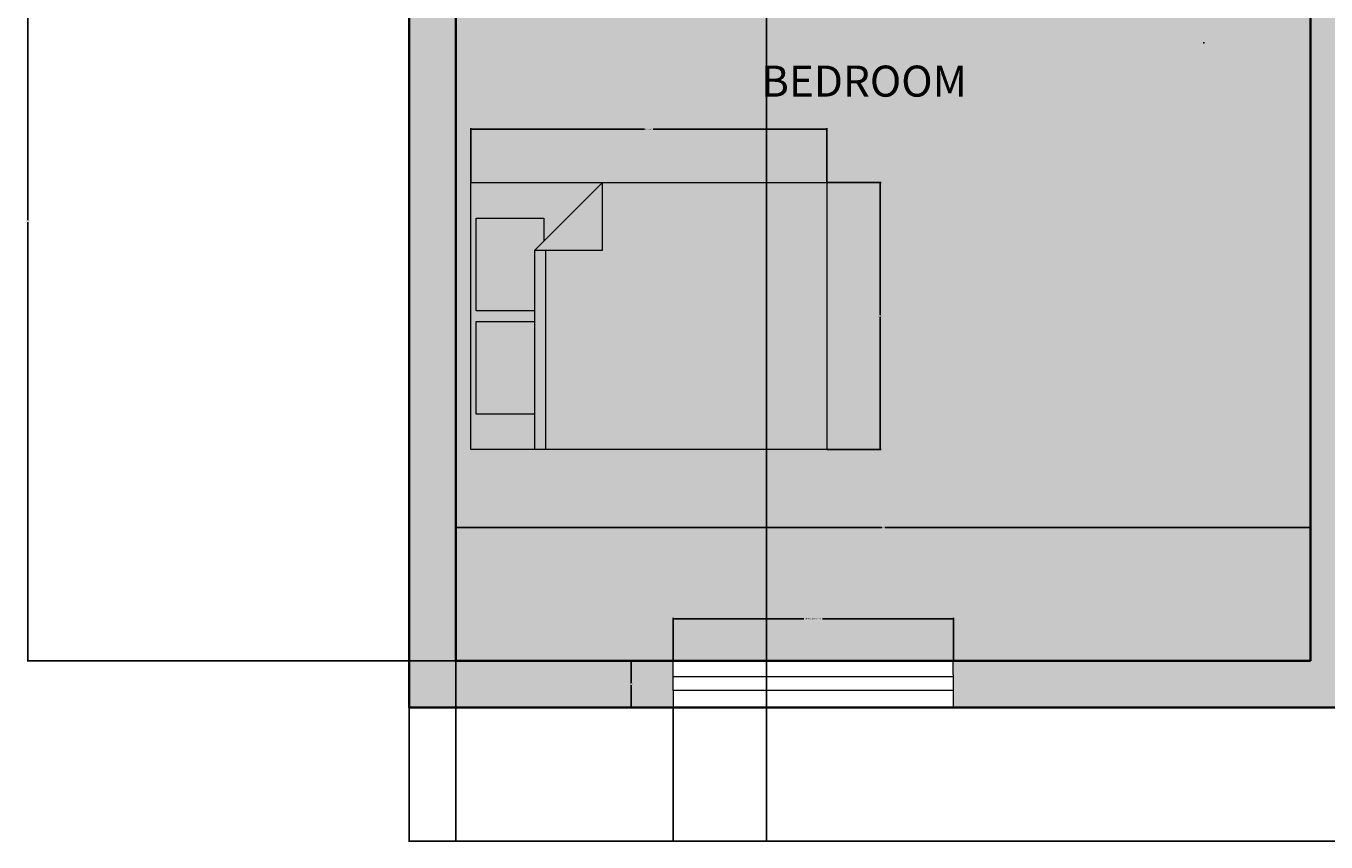
# Model space of a CAD drawing. Units: inches. Extents: x 3024 to 3952, y 1308 to 1863.
# Tile 1 of 29: x 3024 to 3275, y 1322 to 1479. Entities that reach past the tile are written whole.
import ezdxf

# ---------------------------------------------------------------- set-up
doc = ezdxf.new("R2010")
doc.units = ezdxf.units.IN
for name, color, linetype, lineweight in [('A-ANNO-DIMS', 2, 'Continuous', 18), ('A-AREA-IDEN', 7, 'Continuous', 18), ('A-FLOR-TILE-PATT', 7, 'Continuous', 13), ('A-FURN', 8, 'Continuous', 18), ('A-FURN-PATT', 9, 'Continuous', 13), ('A-GLAZ', 4, 'Continuous', 18), ('A-WALL', 7, 'Continuous', 35)]:
    doc.layers.add(name, color=color, linetype=linetype, lineweight=lineweight)
doc.layers.add('A-FLOR-PATT', color=254, linetype='Continuous', lineweight=13, true_color=0xfeeab9)
doc.layers.add('A-WALL-PATT', color=254, linetype='Continuous', lineweight=13, true_color=0xcecce6)
doc.styles.get("Standard").update_dxf_attribs({"font": 'arial.ttf'})
doc.dimstyles.get("Standard").update_dxf_attribs({"dimtxt": 0.18, "dimasz": 0.18, "dimexe": 0.18, "dimexo": 0.0625, "dimgap": 0.09, "dimtad": 0, "dimtih": 1, "dimtoh": 1, "dimdec": 4, "dimzin": 0, "dimdsep": 46, "dimtxsty": 'Standard', "dimcen": 0.09, "dimadec": 0, "dimazin": 0, "dimtfac": 1, "dimtdec": 4, "dimtofl": 0, "dimtmove": 0, "dimatfit": 3, "dimfxl": 1, "dimtolj": 1, "dimtzin": 0, "dimarcsym": 0})

# ---------------------------------------------------------------- blocks, each defined once
blk = doc.blocks.new('Bed - Queen')
for p, q in [((0, -80.00003), (0, 0)), ((0, 0), (59.99999, 0)), ((59.99999, 0), (59.99999, -80.00003)), ((7.99999, -1.2), (28.79998, -1.2)), ((7.99999, -14.4), (7.99999, -1.2)), ((28.79998, -1.2), (28.79998, -14.4)), ((31.19999, -1.2), (51.99999, -1.2)), ((31.19999, -14.4), (31.19999, -1.2)), ((51.99999, -1.2), (51.99999, -16.4)), ((0, -14.4), (44.8, -14.4)), ((59.99999, -29.6), (44.8, -14.4)), ((44.8, -14.4), (44.8, -29.6)), ((44.8, -16.8), (0, -16.8)), ((51.99999, -16.4), (46.79936, -16.4)), ((44.8, -29.6), (59.99999, -29.6)), ((59.99999, -80.00003), (0, -80.00003))]:
    blk.add_line(p, q)
blk = doc.blocks.new('WIN-BEDROOM-54IN')
for p, q in [((0, 5.99), (0, 9)), ((54.08, 6.41), (54.08, 9)), ((54.08, 6.41), (54.08, 5.99)), ((0, 3.28), (0, 0)), ((54.08, 3.69), (54.08, 0))]:
    blk.add_line(p, q)
blk.add_lwpolyline([(0, 5.99), (54.08, 5.99), (54.08, 3.28), (0, 3.28)], close=True)
blk = doc.blocks.new('*D16')
at = {"layer": 'A-ANNO-DIMS', "color": 0, "lineweight": -2, "transparency": 16777216}
for p, q in [((3109.65, 1449.25), (3109.65, 1459.68)), ((3109.83, 1459.5), (3143.2, 1459.5)), ((3178.2, 1459.5), (3144.83, 1459.5)), ((3178.38, 1449.25), (3178.38, 1459.68))]:
    blk.add_line(p, q, dxfattribs=at)
at = {"layer": 'A-ANNO-DIMS', "color": 0, "transparency": 16777216}
for points in [[(3109.83, 1459.53), (3109.83, 1459.47), (3109.65, 1459.5)], [(3178.2, 1459.53), (3178.2, 1459.47), (3178.38, 1459.5)]]:
    blk.add_solid(points, dxfattribs=at)
at = {"layer": 'Defpoints', "color": 0, "transparency": 16777216}
for p in [(3109.65, 1459.5), (3109.65, 1449.19), (3178.38, 1449.19)]:
    blk.add_point(p, dxfattribs=at)
at = {"layer": 'A-ANNO-DIMS', "color": 0, "transparency": 16777216, "insert": (3144.01, 1459.5), "char_height": 0.18, "attachment_point": 5}
blk.add_mtext('\\A1;BED 69 TYP.', dxfattribs=at)
blk = doc.blocks.new('*D17')
at = {"layer": 'A-ANNO-DIMS', "color": 0, "lineweight": -2, "transparency": 16777216}
for p, q in [((3178.44, 1449.19), (3188.87, 1449.19)), ((3188.69, 1449.01), (3188.69, 1423.6)), ((3188.69, 1397.82), (3188.69, 1423.23)), ((3178.44, 1397.64), (3188.87, 1397.64))]:
    blk.add_line(p, q, dxfattribs=at)
at = {"layer": 'A-ANNO-DIMS', "color": 0, "transparency": 16777216}
for points in [[(3188.66, 1449.01), (3188.72, 1449.01), (3188.69, 1449.19)], [(3188.66, 1397.82), (3188.72, 1397.82), (3188.69, 1397.64)]]:
    blk.add_solid(points, dxfattribs=at)
at = {"layer": 'Defpoints', "color": 0, "transparency": 16777216}
for p in [(3178.38, 1449.19), (3188.69, 1449.19), (3178.38, 1397.64)]:
    blk.add_point(p, dxfattribs=at)
at = {"layer": 'A-ANNO-DIMS', "color": 0, "transparency": 16777216, "insert": (3188.69, 1423.41), "char_height": 0.18, "attachment_point": 5}
blk.add_mtext('\\A1;52 TYP.', dxfattribs=at)
blk = doc.blocks.new('*D24')
at = {"layer": 'A-ANNO-DIMS', "color": 0, "lineweight": -2, "transparency": 16777216}
for p, q in [((3148.73, 1356.91), (3148.73, 1365.14)), ((3148.91, 1364.96), (3173.97, 1364.96)), ((3202.63, 1364.96), (3177.56, 1364.96)), ((3202.81, 1356.91), (3202.81, 1365.14))]:
    blk.add_line(p, q, dxfattribs=at)
at = {"layer": 'A-ANNO-DIMS', "color": 0, "transparency": 16777216}
for points in [[(3148.91, 1364.99), (3148.91, 1364.93), (3148.73, 1364.96)], [(3202.63, 1364.99), (3202.63, 1364.93), (3202.81, 1364.96)]]:
    blk.add_solid(points, dxfattribs=at)
at = {"layer": 'Defpoints', "color": 0, "transparency": 16777216}
for p in [(3202.81, 1364.96), (3148.73, 1356.85), (3202.81, 1356.85)]:
    blk.add_point(p, dxfattribs=at)
at = {"layer": 'A-ANNO-DIMS', "color": 0, "transparency": 16777216, "insert": (3175.77, 1364.96), "char_height": 0.18, "attachment_point": 5}
blk.add_mtext('\\A1;BEDROOM WINDOW 54 TYP.', dxfattribs=at)
blk = doc.blocks.new('*D25')
at = {"layer": 'A-ANNO-DIMS', "color": 0, "lineweight": -2, "transparency": 16777216}
for p, q in [((3148.66, 1356.85), (3140.43, 1356.85)), ((3140.61, 1356.67), (3140.61, 1352.53)), ((3140.61, 1348.03), (3140.61, 1352.16)), ((3148.66, 1347.85), (3140.43, 1347.85))]:
    blk.add_line(p, q, dxfattribs=at)
at = {"layer": 'A-ANNO-DIMS', "color": 0, "transparency": 16777216}
for points in [[(3140.58, 1356.67), (3140.64, 1356.67), (3140.61, 1356.85)], [(3140.58, 1348.03), (3140.64, 1348.03), (3140.61, 1347.85)]]:
    blk.add_solid(points, dxfattribs=at)
at = {"layer": 'Defpoints', "color": 0, "transparency": 16777216}
for p in [(3140.61, 1356.85), (3148.73, 1356.85), (3148.73, 1347.85)]:
    blk.add_point(p, dxfattribs=at)
at = {"layer": 'A-ANNO-DIMS', "color": 0, "transparency": 16777216, "insert": (3140.61, 1352.35), "char_height": 0.18, "attachment_point": 5}
blk.add_mtext('\\A1;9 TYP.', dxfattribs=at)
blk = doc.blocks.new('*D36')
at = {"layer": 'A-ANNO-DIMS', "color": 0, "lineweight": -2, "transparency": 16777216}
for p, q in [((3097.76, 1347.78), (3097.76, 1321.89)), ((3469.76, 1347.78), (3469.76, 1321.89)), ((3097.94, 1322.07), (3283.48, 1322.07)), ((3469.58, 1322.07), (3284.05, 1322.07))]:
    blk.add_line(p, q, dxfattribs=at)
at = {"layer": 'A-ANNO-DIMS', "color": 0, "transparency": 16777216}
for points in [[(3097.94, 1322.1), (3097.94, 1322.04), (3097.76, 1322.07)], [(3469.58, 1322.1), (3469.58, 1322.04), (3469.76, 1322.07)]]:
    blk.add_solid(points, dxfattribs=at)
at = {"layer": 'Defpoints', "color": 0, "transparency": 16777216}
for p in [(3097.76, 1347.85), (3469.76, 1347.85), (3469.76, 1322.07)]:
    blk.add_point(p, dxfattribs=at)
at = {"layer": 'A-ANNO-DIMS', "color": 0, "transparency": 16777216, "insert": (3283.76, 1322.07), "char_height": 0.18, "attachment_point": 5}
blk.add_mtext('\\A1;372', dxfattribs=at)
blk = doc.blocks.new('*D44')
at = {"layer": 'A-ANNO-DIMS', "color": 0, "lineweight": -2, "transparency": 16777216}
for p, q in [((3106.7, 1526.61), (3023.95, 1526.61)), ((3024.13, 1526.43), (3024.13, 1441.91)), ((3024.13, 1357.03), (3024.13, 1441.54)), ((3106.7, 1356.85), (3023.95, 1356.85))]:
    blk.add_line(p, q, dxfattribs=at)
at = {"layer": 'A-ANNO-DIMS', "color": 0, "transparency": 16777216}
for points in [[(3024.1, 1526.43), (3024.16, 1526.43), (3024.13, 1526.61)], [(3024.1, 1357.03), (3024.16, 1357.03), (3024.13, 1356.85)]]:
    blk.add_solid(points, dxfattribs=at)
at = {"layer": 'Defpoints', "color": 0, "transparency": 16777216}
for p in [(3106.76, 1526.61), (3024.13, 1356.85), (3106.76, 1356.85)]:
    blk.add_point(p, dxfattribs=at)
at = {"layer": 'A-ANNO-DIMS', "color": 0, "transparency": 16777216, "insert": (3024.13, 1441.73), "char_height": 0.18, "attachment_point": 5}
blk.add_mtext('\\A1;169.76', dxfattribs=at)
blk = doc.blocks.new('*D45')
at = {"layer": 'A-ANNO-DIMS', "color": 0, "lineweight": -2, "transparency": 16777216}
for p, q in [((3106.76, 1356.91), (3106.76, 1382.8)), ((3106.94, 1382.62), (3188.98, 1382.62)), ((3271.58, 1382.62), (3189.55, 1382.62)), ((3271.76, 1356.91), (3271.76, 1382.8))]:
    blk.add_line(p, q, dxfattribs=at)
at = {"layer": 'A-ANNO-DIMS', "color": 0, "transparency": 16777216}
for points in [[(3106.94, 1382.65), (3106.94, 1382.59), (3106.76, 1382.62)], [(3271.58, 1382.65), (3271.58, 1382.59), (3271.76, 1382.62)]]:
    blk.add_solid(points, dxfattribs=at)
at = {"layer": 'Defpoints', "color": 0, "transparency": 16777216}
for p in [(3271.76, 1382.62), (3106.76, 1356.85), (3271.76, 1356.85)]:
    blk.add_point(p, dxfattribs=at)
at = {"layer": 'A-ANNO-DIMS', "color": 0, "transparency": 16777216, "insert": (3189.26, 1382.62), "char_height": 0.18, "attachment_point": 5}
blk.add_mtext('\\A1;165', dxfattribs=at)
blk = doc.blocks.new('*D47')
at = {"layer": 'A-ANNO-DIMS', "color": 0, "lineweight": -2, "transparency": 16777216}
for p, q in [((3106.76, 1628.54), (3106.76, 1321.89)), ((3166.76, 1628.54), (3166.76, 1321.89)), ((3106.94, 1322.07), (3136.54, 1322.07)), ((3166.58, 1322.07), (3136.98, 1322.07))]:
    blk.add_line(p, q, dxfattribs=at)
at = {"layer": 'A-ANNO-DIMS', "color": 0, "transparency": 16777216}
for points in [[(3106.94, 1322.1), (3106.94, 1322.04), (3106.76, 1322.07)], [(3166.58, 1322.1), (3166.58, 1322.04), (3166.76, 1322.07)]]:
    blk.add_solid(points, dxfattribs=at)
at = {"layer": 'Defpoints', "color": 0, "transparency": 16777216}
for p in [(3106.76, 1628.61), (3166.76, 1628.61), (3166.76, 1322.07)]:
    blk.add_point(p, dxfattribs=at)
at = {"layer": 'A-ANNO-DIMS', "color": 0, "transparency": 16777216, "insert": (3136.76, 1322.07), "char_height": 0.18, "attachment_point": 5}
blk.add_mtext('\\A1;60', dxfattribs=at)
blk = doc.blocks.new('*D75')
at = {"layer": 'A-ANNO-DIMS', "color": 0, "lineweight": -2, "transparency": 16777216}
for p, q in [((3097.76, 1347.78), (3097.76, 1321.89)), ((3148.73, 1347.78), (3148.73, 1321.89)), ((3097.94, 1322.07), (3122.85, 1322.07)), ((3148.55, 1322.07), (3123.64, 1322.07))]:
    blk.add_line(p, q, dxfattribs=at)
at = {"layer": 'A-ANNO-DIMS', "color": 0, "transparency": 16777216}
for points in [[(3097.94, 1322.1), (3097.94, 1322.04), (3097.76, 1322.07)], [(3148.55, 1322.1), (3148.55, 1322.04), (3148.73, 1322.07)]]:
    blk.add_solid(points, dxfattribs=at)
at = {"layer": 'Defpoints', "color": 0, "transparency": 16777216}
for p in [(3097.76, 1347.85), (3148.73, 1347.85), (3097.76, 1322.07)]:
    blk.add_point(p, dxfattribs=at)
at = {"layer": 'A-ANNO-DIMS', "color": 0, "transparency": 16777216, "insert": (3123.25, 1322.07), "char_height": 0.18, "attachment_point": 5}
blk.add_mtext('\\A1;50.96', dxfattribs=at)
blk = doc.blocks.new('*D106')
at = {"layer": 'A-ANNO-DIMS', "color": 0, "lineweight": -2, "transparency": 16777216}
for p, q in [((3251.11, 1476.18), (3251.29, 1476.18)), ((3251.2, 1476.09), (3251.2, 1476.27)), ((3316.02, 1476.18), (3291.89, 1476.18))]:
    blk.add_line(p, q, dxfattribs=at)
at = {"layer": 'A-ANNO-DIMS', "color": 0, "transparency": 16777216}
blk.add_solid([(3291.89, 1476.21), (3291.89, 1476.15), (3291.71, 1476.18)], dxfattribs=at)
at = {"layer": 'Defpoints', "color": 0, "transparency": 16777216}
for p in [(3251.2, 1476.18), (3291.71, 1476.18)]:
    blk.add_point(p, dxfattribs=at)
at = {"layer": 'A-ANNO-DIMS', "color": 0, "transparency": 16777216, "insert": (3316.48, 1476.18), "char_height": 0.18, "attachment_point": 5}
blk.add_mtext('\\A1;R40.51', dxfattribs=at)

msp = doc.modelspace()

# ---------------------------------------------------------------- hatches: boundary and pattern name
at = {"layer": 'A-FLOR-PATT', "transparency": 33554528}
h = msp.add_hatch(color=256, dxfattribs=at)
h.dxf.hatch_style = 1
h.paths.add_polyline_path([(3460.764, 1688.6064), (3412.764, 1688.6064), (3412.764, 1694.6064), (3460.764, 1694.6064), (3460.764, 1778.6064), (3406.764, 1778.6064), (3406.764, 1759.9514), (3318.2981, 1759.9514), (3318.2981, 1658.6064), (3322.5356, 1658.6064), (3322.5356, 1652.6064), (3292.764, 1652.6064), (3292.764, 1778.6064), (3106.764, 1778.6064), (3106.764, 1628.6064), (3172.764, 1628.6064), (3172.764, 1532.6064), (3166.764, 1532.6064), (3166.764, 1628.6064), (3106.764, 1628.6064), (3106.764, 1356.8452), (3202.812, 1356.8452), (3202.812, 1354.2534), (3202.812, 1353.8388), (3202.812, 1351.1212), (3202.812, 1347.8452), (3277.764, 1347.8452), (3277.764, 1353.8452), (3277.764, 1356.8452), (3277.764, 1442.6064), (3460.764, 1442.6064)])
h.paths.add_polyline_path([(3216.238, 1527.2064), (3216.238, 1491.2064), (3214.663, 1491.2064), (3214.663, 1491.2409, -0.39662236), (3180.243, 1526.6064), (3163.0285, 1526.6064), (3163.0285, 1531.1064), (3161.716, 1531.1064), (3161.716, 1561.1064), (3163.0285, 1561.1064), (3163.0285, 1531.1064), (3163.0285, 1526.6064), (3180.243, 1526.6064, 0.39662236), (3214.663, 1491.2409), (3214.663, 1527.2064)], flags=16)
h.paths.add_polyline_path([(3227.364, 1649.8972), (3191.364, 1649.8972), (3191.364, 1651.4722), (3227.364, 1651.4722)], flags=16)
h.paths.add_polyline_path([(3323.1172, 1606.7362), (3323.8545, 1606.8514), (3323.8545, 1594.8241), (3323.1172, 1594.9393)], flags=16)
h.paths.add_polyline_path([(3324.2232, 1606.909), (3330.1216, 1607.8307), (3330.1216, 1614.1093), (3339.3495, 1614.1093), (3340.2711, 1620.0078), (3352.4136, 1620.0078), (3353.3353, 1614.1093), (3359.9941, 1614.1093), (3360.9157, 1620.0078), (3373.0582, 1620.0078), (3373.9799, 1614.1093), (3383.2077, 1614.1093), (3383.2077, 1607.8307), (3389.1062, 1606.909), (3389.1062, 1594.7665), (3383.2077, 1593.8449), (3383.2077, 1587.5663), (3373.9799, 1587.5663), (3373.0583, 1581.6678), (3360.9157, 1581.6678), (3359.9941, 1587.5663), (3353.3353, 1587.5663), (3352.4136, 1581.6678), (3340.2711, 1581.6678), (3339.3495, 1587.5663), (3330.1216, 1587.5663), (3330.1216, 1593.8449), (3324.2232, 1594.7665)], flags=16)
h.paths.add_polyline_path([(3236.1584, 1693.1064), (3236.1584, 1723.1064), (3237.4709, 1723.1064), (3237.4709, 1693.1064)], flags=16)
h.paths.add_polyline_path([(3373.2158, 1600.6847), (3373.7965, 1600.7303), (3374.3268, 1600.7874), (3374.8132, 1600.8531), (3375.2621, 1600.9247), (3375.6801, 1600.9991), (3376.0736, 1601.0735), (3376.6855, 1601.19), (3377.366, 1601.3023), (3378.0667, 1601.3814), (3378.8026, 1601.4123), (3379.5865, 1601.3839), (3380.4537, 1601.2948), (3381.301, 1601.1717), (3382.0317, 1601.0433), (3382.4398, 1600.9607), (3382.6252, 1600.9201), (3382.919, 1600.8507), (3382.9044, 1600.8531), (3382.842, 1600.8678), (3382.7541, 1600.8896), (3382.6252, 1600.9201), (3382.4398, 1600.9607), (3382.1868, 1601.0119), (3381.8738, 1601.0711), (3381.5125, 1601.1346), (3381.1149, 1601.1988), (3380.6928, 1601.2601), (3380.2581, 1601.3149), (3379.8226, 1601.3597), (3379.3984, 1601.3908), (3378.9944, 1601.4054), (3378.6092, 1601.4042), (3378.2384, 1601.3886), (3377.8777, 1601.36), (3377.5227, 1601.32), (3377.1691, 1601.2698), (3376.8127, 1601.211), (3376.4491, 1601.145), (3376.0736, 1601.0735), (3375.4177, 1600.9494), (3374.5542, 1600.8119), (3373.5044, 1600.6988)], flags=0)
h.paths.add_polyline_path([(3380.0253, 1596.7351), (3380.499, 1596.6659), (3380.9706, 1596.6119), (3381.4375, 1596.5791), (3381.8971, 1596.5736), (3382.5886, 1596.6167), (3382.7848, 1596.6692), (3382.1465, 1596.5706), (3381.236, 1596.5815), (3380.3199, 1596.6865)], flags=0)
h.paths.add_polyline_path([(3369.6414, 1603.9617), (3370.1589, 1604.0021), (3370.6218, 1604.0539), (3371.0335, 1604.1173), (3371.3978, 1604.1921), (3371.7181, 1604.2785), (3371.9984, 1604.3761), (3372.2441, 1604.483), (3372.4611, 1604.5972), (3372.655, 1604.7163), (3372.8317, 1604.8384), (3372.9968, 1604.9611), (3373.3703, 1605.2455), (3373.8426, 1605.5328), (3374.4624, 1605.7539), (3375.1058, 1605.8302), (3375.7221, 1605.8261), (3376.4109, 1605.76), (3377.1534, 1605.6376), (3377.8945, 1605.473), (3378.1382, 1605.409), (3377.7394, 1605.5074), (3377.3509, 1605.5937), (3376.9704, 1605.6677), (3376.5999, 1605.7288), (3376.2417, 1605.7762), (3375.8979, 1605.8092), (3375.5707, 1605.8271), (3375.2621, 1605.8291), (3374.9745, 1605.8146), (3374.7092, 1605.7832), (3374.4647, 1605.7359), (3374.239, 1605.6742), (3374.0298, 1605.5996), (3373.835, 1605.5134), (3373.6525, 1605.4171), (3373.4801, 1605.3123), (3373.3156, 1605.2002), (3373.1562, 1605.0825), (3372.7603, 1604.781), (3372.236, 1604.4588), (3371.5738, 1604.2283), (3370.8493, 1604.0794), (3369.9262, 1603.976)], flags=0)
h.paths.add_polyline_path([(3366.7533, 1606.5832), (3367.1713, 1606.5519), (3367.5378, 1606.5374), (3367.8568, 1606.5394), (3368.1325, 1606.5573), (3368.3694, 1606.5903), (3368.5717, 1606.6377), (3368.7438, 1606.6988), (3368.89, 1606.7728), (3369.0146, 1606.8591), (3369.121, 1606.9568), (3369.2094, 1607.0646), (3369.2792, 1607.181), (3369.3295, 1607.3046), (3369.3596, 1607.4339), (3369.3688, 1607.5676), (3369.3565, 1607.7042), (3369.3218, 1607.8422), (3369.2649, 1607.9804), (3369.1893, 1608.1187), (3369.0993, 1608.2569), (3368.9992, 1608.3952), (3368.8934, 1608.5334), (3368.7861, 1608.6717), (3368.6817, 1608.8099), (3368.4212, 1609.1804), (3368.2685, 1609.7106), (3368.4883, 1610.1814), (3369.0537, 1610.4604), (3369.6717, 1610.5097), (3370.2812, 1610.3612), (3370.4805, 1610.2968), (3370.1882, 1610.3839), (3369.9284, 1610.4472), (3369.6905, 1610.4842), (3369.4662, 1610.4933), (3369.2555, 1610.4765), (3369.0608, 1610.4367), (3368.884, 1610.3767), (3368.7274, 1610.2994), (3368.5931, 1610.2077), (3368.4833, 1610.1045), (3368.4002, 1609.9927), (3368.3451, 1609.8747), (3368.3166, 1609.7517), (3368.3127, 1609.6244), (3368.331, 1609.4935), (3368.3696, 1609.3597), (3368.4261, 1609.2237), (3368.4985, 1609.0863), (3368.5845, 1608.9482), (3368.6817, 1608.8099), (3368.7861, 1608.6717), (3368.8934, 1608.5334), (3368.9992, 1608.3952), (3369.0993, 1608.2569), (3369.3398, 1607.8876), (3369.3941, 1607.2896), (3368.9774, 1606.7817), (3368.3928, 1606.5742), (3367.7162, 1606.5303), (3367.0044, 1606.5585)], flags=0)
h.paths.add_polyline_path([(3362.1859, 1610.2589), (3362.5478, 1610.2845), (3362.8348, 1610.3275), (3363.0585, 1610.3863), (3363.2303, 1610.4595), (3363.3619, 1610.5457), (3363.463, 1610.6432), (3363.5376, 1610.7502), (3363.5876, 1610.8643), (3363.6153, 1610.9834), (3363.6229, 1611.1055), (3363.6125, 1611.2283), (3363.5861, 1611.3496), (3363.5462, 1611.4673), (3363.4949, 1611.5797), (3363.4358, 1611.6871), (3363.3723, 1611.7902), (3363.3081, 1611.8897), (3363.2468, 1611.9863), (3363.192, 1612.0808), (3363.0258, 1612.4261), (3363.3371, 1612.8672), (3363.9008, 1612.9782), (3364.4822, 1612.9641), (3365.1098, 1612.9074), (3365.328, 1612.8805), (3364.9615, 1612.9208), (3364.6426, 1612.9496), (3364.3668, 1612.9669), (3364.1299, 1612.9726), (3363.9276, 1612.9669), (3363.7555, 1612.9496), (3363.6093, 1612.9208), (3363.4848, 1612.8805), (3363.3782, 1612.8289), (3363.2889, 1612.7672), (3363.2169, 1612.6969), (3363.1622, 1612.6193), (3363.1247, 1612.5361), (3363.1046, 1612.4484), (3363.1017, 1612.358), (3363.1161, 1612.266), (3363.1472, 1612.1738), (3363.192, 1612.0808), (3363.2468, 1611.9863), (3363.3081, 1611.8897), (3363.3723, 1611.7902), (3363.4358, 1611.6871), (3363.6363, 1611.323), (3363.5979, 1610.7003), (3363.0863, 1610.3651), (3362.3983, 1610.2622)], flags=0)
h.paths.add_polyline_path([(3352.356, 1581.2991), (3352.2408, 1580.5618), (3340.4439, 1580.5618), (3340.3287, 1581.2991)], flags=16)
h.paths.add_polyline_path([(3340.4439, 1621.1137), (3352.2408, 1621.1137), (3352.356, 1620.3764), (3340.3287, 1620.3764)], flags=16)
h.paths.add_polyline_path([(3278.4282, 1504.7424), (3290.3831, 1504.7424), (3290.3831, 1502.7499), (3291.0473, 1502.7499), (3291.0473, 1494.7799), (3290.3831, 1494.7799), (3290.3831, 1494.1158), (3291.0473, 1494.1158), (3291.0473, 1486.1458), (3290.3831, 1486.1458), (3290.3831, 1484.1533), (3291.0473, 1484.1533), (3291.0473, 1483.4892, -0.09090909), (3291.0473, 1468.8776), (3291.0473, 1468.2135), (3290.3831, 1468.2135), (3290.3831, 1464.8926), (3278.4282, 1464.8926), (3278.4282, 1472.8626), (3277.764, 1473.5268), (3277.764, 1478.84), (3278.4282, 1479.5042)], flags=16)
h.paths.add_polyline_path([(3278.7603, 1504.4103), (3290.051, 1504.4103), (3290.051, 1465.2247), (3278.7603, 1465.2247)], flags=0)
h.paths.add_polyline_path([(3123.904, 1600.7821), (3117.9039, 1602.7821), (3117.9039, 1599.7821), (3119.4039, 1599.7821), (3119.4039, 1596.7821), (3118.4039, 1596.7821), (3118.4039, 1598.7821), (3117.9039, 1598.7821), (3117.9039, 1596.2821), (3109.9039, 1596.2821), (3109.9039, 1617.2821), (3117.9039, 1617.2821), (3117.9039, 1610.7821), (3123.9038, 1612.7821, -0.70257121), (3137.9039, 1606.7822, -0.70256205)], flags=16)
h.paths.add_polyline_path([(3123.9039, 1602.7822), (3123.9039, 1610.7822, -0.73453329), (3136.9039, 1606.7822, -0.73452973)], flags=0)
h.paths.add_polyline_path([(3177.972, 1689.6473), (3109.2405, 1689.6473), (3109.2405, 1741.1959), (3177.972, 1741.1959)], flags=16)
h.paths.add_polyline_path([(3373.0006, 1581.2991), (3372.8854, 1580.5618), (3361.0885, 1580.5618), (3360.9733, 1581.2991)], flags=16)
h.paths.add_polyline_path([(3361.0885, 1621.1137), (3372.8854, 1621.1137), (3373.0006, 1620.3764), (3360.9733, 1620.3764)], flags=16)
h.paths.add_polyline_path([(3116.9039, 1598.2821, -0.41421356), (3116.1539, 1597.2821), (3111.9039, 1597.2821, -0.41421356), (3110.9039, 1598.0321), (3110.9039, 1615.2821, -0.41421356), (3111.6539, 1616.2821), (3115.9039, 1616.2821, -0.41421356), (3116.9039, 1615.5321)], flags=0)
h.paths.add_polyline_path([(3121.6122, 1728.1369), (3121.6122, 1696.5205), (3110.2715, 1696.5205), (3110.2715, 1714.3906), (3121.6122, 1714.3906), (3121.6122, 1716.4526), (3110.2715, 1716.4526), (3110.2715, 1734.3228), (3123.3304, 1734.3228), (3123.3304, 1729.8552), (3134.6711, 1741.1959), (3134.6711, 1728.1369)], flags=0)
h.paths.add_polyline_path([(3389.4748, 1606.8514), (3390.2122, 1606.7362), (3390.2122, 1594.9393), (3389.4748, 1594.8241)], flags=16)
h.paths.add_polyline_path([(3257.6842, 1762.8281), (3259.6842, 1768.8281), (3256.6842, 1768.8281), (3256.6842, 1767.3281), (3253.6842, 1767.3281), (3253.6842, 1768.3281), (3255.6842, 1768.3281), (3255.6842, 1768.8281), (3253.1842, 1768.8281), (3253.1842, 1776.8281), (3274.1842, 1776.8281), (3274.1842, 1768.8281), (3267.6842, 1768.8281), (3269.6842, 1762.8282, -0.70257121), (3263.6843, 1748.8282, -0.70256205)], flags=16)
h.paths.add_polyline_path([(3259.6842, 1762.8281), (3267.6843, 1762.8281, -0.73453329), (3263.6842, 1749.8282, -0.73452973)], flags=0)
h.paths.add_polyline_path([(3411.264, 1715.6064), (3411.264, 1716.9189), (3441.264, 1716.9189), (3441.264, 1715.6064)], flags=16)
h.paths.add_polyline_path([(3178.3806, 1449.1876), (3178.3806, 1397.639), (3109.6491, 1397.639), (3109.6491, 1449.1876)], flags=16)
h.paths.add_polyline_path([(3397.1501, 1541.7146), (3419.6183, 1541.7146), (3419.6183, 1496.7783), (3397.1501, 1496.7783)], flags=16)
h.paths.add_polyline_path([(3254.1842, 1770.5781), (3254.1842, 1774.8281, -0.41421356), (3254.9342, 1775.8281), (3272.1842, 1775.8281, -0.41421356), (3273.1842, 1775.0781), (3273.1842, 1770.8281, -0.41421356), (3272.4342, 1769.8281), (3255.1842, 1769.8281, -0.41421356)], flags=0)
h.paths.add_polyline_path([(3403.672, 1500.7601), (3403.6016, 1500.3997), (3403.5328, 1500.0441), (3403.4662, 1499.6867), (3403.4027, 1499.3226), (3403.3464, 1498.9532), (3403.3025, 1498.5811), (3403.2759, 1498.2091), (3403.2714, 1497.8401), (3403.3064, 1497.2813), (3403.3491, 1497.1219), (3403.2689, 1497.6395), (3403.2778, 1498.3719), (3403.3635, 1499.0984), (3403.4889, 1499.8168), (3403.6016, 1500.3997), (3403.672, 1500.7601), (3403.744, 1501.1315), (3403.817, 1501.5205), (3403.891, 1501.9336), (3403.9656, 1502.3769), (3404.0404, 1502.8572), (3404.115, 1503.3786), (3404.2264, 1504.2311), (3404.2571, 1504.5223), (3404.1552, 1503.6598), (3404.0063, 1502.6193), (3403.8604, 1501.7518), (3403.744, 1501.1315)], flags=0)
h.paths.add_polyline_path([(3406.5868, 1505.0416), (3406.6121, 1504.5236), (3406.6492, 1504.0526), (3406.6956, 1503.624), (3406.7491, 1503.2333), (3406.8072, 1502.8759), (3406.8676, 1502.5473), (3406.9281, 1502.243), (3407.0268, 1501.7597), (3407.1416, 1501.1368), (3407.2087, 1500.3904), (3407.1804, 1499.6703), (3407.1078, 1498.9956), (3407.0074, 1498.3199), (3406.8809, 1497.6059), (3406.7403, 1496.9627), (3406.7418, 1496.9824), (3406.7491, 1497.0249), (3406.8229, 1497.3409), (3406.8364, 1497.4025), (3406.878, 1497.6078), (3406.9261, 1497.8614), (3406.9777, 1498.1526), (3407.0298, 1498.4712), (3407.0797, 1498.8068), (3407.1243, 1499.149), (3407.1607, 1499.4874), (3407.1859, 1499.8115), (3407.1978, 1500.1137), (3407.1969, 1500.3962), (3407.1841, 1500.6642), (3407.1609, 1500.9225), (3407.1284, 1501.1761), (3407.0876, 1501.43), (3407.0398, 1501.6891), (3406.9862, 1501.9585), (3406.8832, 1502.4628), (3406.7712, 1503.0713), (3406.6657, 1503.8424), (3406.5924, 1504.7735)], flags=0)
h.paths.add_polyline_path([(3409.2517, 1507.8962), (3409.2752, 1507.4282), (3409.3079, 1507.0076), (3409.3501, 1506.6314), (3409.4015, 1506.2969), (3409.4624, 1506.0009), (3409.5326, 1505.7406), (3409.6119, 1505.5128), (3409.6988, 1505.3131), (3409.7915, 1505.1368), (3409.8883, 1504.9792), (3409.9875, 1504.8356), (3410.0872, 1504.7015), (3410.1859, 1504.572), (3410.4508, 1504.2132), (3410.7205, 1503.6035), (3410.8059, 1502.8824), (3410.7619, 1502.0875), (3410.6122, 1501.2299), (3410.4402, 1500.6169), (3410.2538, 1500.0031), (3410.0536, 1499.3219), (3409.9909, 1499.0812), (3410.1761, 1499.7472), (3410.3596, 1500.3513), (3410.4512, 1500.6561), (3410.5312, 1500.9412), (3410.6013, 1501.226), (3410.6614, 1501.512), (3410.7111, 1501.7964), (3410.7496, 1502.0763), (3410.7764, 1502.3489), (3410.7909, 1502.6114), (3410.7926, 1502.8608), (3410.7808, 1503.0944), (3410.7553, 1503.31), (3410.7169, 1503.5087), (3410.6667, 1503.6921), (3410.6061, 1503.8621), (3410.5361, 1504.0203), (3410.4578, 1504.1686), (3410.3726, 1504.3088), (3410.2815, 1504.4424), (3410.1859, 1504.572), (3410.0872, 1504.7015), (3409.859, 1505.0083), (3409.5943, 1505.5117), (3409.4266, 1506.1336), (3409.324, 1506.8011), (3409.2586, 1507.6407)], flags=0)
h.paths.add_polyline_path([(3411.4914, 1510.5878), (3411.4432, 1510.1586), (3411.4054, 1509.775), (3411.38, 1509.4354), (3411.3681, 1509.1376), (3411.3698, 1508.8784), (3411.3843, 1508.6542), (3411.4112, 1508.4618), (3411.4497, 1508.2974), (3411.4994, 1508.1575), (3411.5595, 1508.0388), (3411.6296, 1507.9375), (3411.7097, 1507.851), (3411.802, 1507.7792), (3411.9096, 1507.7225), (3412.0353, 1507.6817), (3412.1821, 1507.6572), (3412.3528, 1507.6496), (3412.5505, 1507.6597), (3412.778, 1507.6879), (3413.0364, 1507.7341), (3413.3194, 1507.7955), (3413.6188, 1507.8687), (3413.9264, 1507.95), (3414.234, 1508.036), (3414.5333, 1508.1232), (3414.8163, 1508.208), (3415.0747, 1508.287), (3415.3023, 1508.3569), (3415.5007, 1508.4158), (3415.6733, 1508.4617), (3416.1158, 1508.5538), (3416.512, 1508.2591), (3416.716, 1507.6581), (3416.61, 1507.0003), (3416.3052, 1506.3411), (3415.8928, 1505.618), (3415.7339, 1505.3633), (3415.9914, 1505.791), (3416.201, 1506.1583), (3416.3666, 1506.4739), (3416.4925, 1506.7462), (3416.5828, 1506.9838), (3416.6413, 1507.1949), (3416.6725, 1507.3883), (3416.6799, 1507.5705), (3416.6662, 1507.7417), (3416.6339, 1507.9), (3416.5851, 1508.0436), (3416.5223, 1508.1709), (3416.4478, 1508.28), (3416.3639, 1508.3692), (3416.273, 1508.4368), (3416.1765, 1508.4815), (3416.0718, 1508.5047), (3415.9553, 1508.5079), (3415.8237, 1508.493), (3415.6733, 1508.4617), (3415.5007, 1508.4158), (3415.3327, 1508.3659), (3414.6495, 1508.157), (3414.0606, 1507.9855), (3413.4456, 1507.8229), (3412.8838, 1507.701), (3412.5505, 1507.6597), (3412.0748, 1507.6354), (3411.595, 1507.8883), (3411.398, 1508.4429), (3411.3624, 1508.9927), (3411.3854, 1509.5711), (3411.4578, 1510.3071)], flags=0)
h.paths.add_polyline_path([(3135.0797, 1449.1876), (3135.0797, 1436.1286), (3122.0208, 1436.1286), (3122.0208, 1404.5122), (3110.6801, 1404.5122), (3110.6801, 1422.3823), (3122.0208, 1422.3823), (3122.0208, 1424.4443), (3110.6801, 1424.4443), (3110.6801, 1442.3145), (3123.739, 1442.3145), (3123.739, 1437.8469)], flags=0)
h.paths.add_polyline_path([(3416.4944, 1514.2949), (3416.4837, 1513.8511), (3416.4893, 1513.4867), (3416.5102, 1513.1926), (3416.5451, 1512.9593), (3416.5929, 1512.7775), (3416.6524, 1512.6379), (3416.7224, 1512.531), (3416.8017, 1512.4488), (3416.8886, 1512.3882), (3416.9813, 1512.3476), (3417.0781, 1512.3251), (3417.1773, 1512.3189), (3417.277, 1512.3274), (3417.3757, 1512.3488), (3417.4713, 1512.3813), (3417.5627, 1512.4229), (3417.65, 1512.471), (3417.7338, 1512.5225), (3417.8146, 1512.5747), (3417.8931, 1512.6245), (3417.9699, 1512.6691), (3418.2968, 1512.8265), (3418.6505, 1512.4645), (3418.7037, 1511.9342), (3418.6693, 1511.3839), (3418.6076, 1510.8228), (3418.5777, 1510.5927), (3418.6197, 1510.9333), (3418.6525, 1511.2311), (3418.6759, 1511.4903), (3418.6899, 1511.7144), (3418.6946, 1511.9069), (3418.6899, 1512.0713), (3418.6759, 1512.2112), (3418.6525, 1512.33), (3418.6197, 1512.4311), (3418.5778, 1512.5177), (3418.5276, 1512.5903), (3418.4705, 1512.6488), (3418.4075, 1512.6933), (3418.3399, 1512.7237), (3418.2686, 1512.7401), (3418.1951, 1512.7424), (3418.1204, 1512.7307), (3418.0455, 1512.7055), (3417.9792, 1512.6736), (3417.65, 1512.471), (3417.5627, 1512.4229), (3417.4713, 1512.3813), (3417.3757, 1512.3488), (3417.277, 1512.3274), (3416.878, 1512.2936), (3416.5757, 1512.7549), (3416.492, 1513.3145), (3416.4808, 1514.0384)], flags=0)
h.paths.add_polyline_path([(3392.8223, 1481.9454), (3396.7707, 1481.9454), (3396.7707, 1480.9201), (3428.3585, 1480.9201), (3428.3585, 1481.9454), (3432.3069, 1481.9454), (3432.3069, 1464.8354, -0.26666697), (3392.8223, 1464.8354)], flags=16)
h.paths.add_polyline_path([(3431.203, 1547.5428), (3450.8613, 1547.5428, -0.19047621), (3450.8614, 1484.031), (3431.203, 1484.031), (3431.203, 1488.5675), (3432.3809, 1488.5675), (3432.3809, 1543.0062), (3431.203, 1543.0062)], flags=16)
h.paths.add_polyline_path([(3451.9233, 1524.86, -0.04962821), (3451.9233, 1506.7138), (3446.7921, 1506.7138), (3446.7921, 1524.86)], flags=0)
h.paths.add_polyline_path([(3460.764, 1436.6064), (3277.764, 1436.6064), (3277.764, 1356.8452), (3277.764, 1353.8452), (3460.764, 1353.8452)], flags=17)
h.paths.add_polyline_path([(3121.3033, 1577.378), (3153.693, 1577.378), (3153.693, 1586.6752), (3121.3033, 1586.6752)], flags=24)
h.paths.add_polyline_path([(3164.1457, 1464.1276), (3210.4801, 1464.1276), (3210.4801, 1473.4247), (3164.1457, 1473.4247)], flags=24)
h.paths.add_polyline_path([(3343.1909, 1505.8863), (3373.7236, 1505.8863), (3373.7236, 1515.1773), (3343.1909, 1515.1773)], flags=24)
h.paths.add_polyline_path([(3337.6353, 1564.2926), (3370.0189, 1564.2926), (3370.0189, 1573.5836), (3337.6353, 1573.5836)], flags=24)
h.paths.add_polyline_path([(3419.204, 1753.8578), (3453.3997, 1753.8578), (3453.3997, 1762.9956), (3419.204, 1762.9956)], flags=24)
h.paths.add_polyline_path([(3341.2523, 1701.0246), (3381.0761, 1701.0246), (3381.0761, 1710.3156), (3341.2523, 1710.3156)], flags=24)
h.paths.add_polyline_path([(3245.8895, 1726.2997), (3278.2793, 1726.2997), (3278.2793, 1735.5968), (3245.8895, 1735.5968)], flags=24)
h.paths.add_polyline_path([(3128.8045, 1668.6736), (3175.1389, 1668.6736), (3175.1389, 1677.9707), (3128.8045, 1677.9707)], flags=24)
h.paths.add_polyline_path([(3345.9997, 1396.0062), (3389.09, 1396.0062), (3389.09, 1405.3033), (3345.9997, 1405.3033)], flags=24)
at = {"layer": 'A-FLOR-TILE-PATT', "transparency": 33554569}
h = msp.add_hatch(dxfattribs=at)
h.set_pattern_fill('ANGLE', color=256, scale=2)
h.set_pattern_definition([(0, (0, 0), (0, 13.97), [10.16, -3.81]), (90, (0, 0), (-13.97, 9e-16), [10.16, -3.81])])
h.paths.add_polyline_path([(3292.764, 1778.6064), (3232.764, 1778.6064), (3232.764, 1694.6064), (3236.1584, 1694.6064), (3236.1584, 1723.1064), (3237.4709, 1723.1064), (3237.4709, 1723.0777, -0.38700389), (3266.1209, 1694.6064), (3292.764, 1694.6064)])
h.paths.add_polyline_path([(3263.6843, 1748.8282, -0.70256205), (3257.6842, 1762.8281), (3259.6842, 1768.8281), (3256.6842, 1768.8281), (3256.6842, 1767.3281), (3253.6842, 1767.3281), (3253.6842, 1768.3281), (3255.6842, 1768.3281), (3255.6842, 1768.8281), (3253.1842, 1768.8281), (3253.1842, 1776.8281), (3274.1842, 1776.8281), (3274.1842, 1768.8281), (3267.6842, 1768.8281), (3269.6842, 1762.8282, -0.70257121)], flags=16)
h.paths.add_polyline_path([(3263.6842, 1749.8282, -0.73452973), (3259.6842, 1762.8281), (3267.6843, 1762.8281, -0.73453329)], flags=0)
h.paths.add_polyline_path([(3255.1842, 1769.8281, -0.41421356), (3254.1842, 1770.5781), (3254.1842, 1774.8281, -0.41421356), (3254.9342, 1775.8281), (3272.1842, 1775.8281, -0.41421356), (3273.1842, 1775.0781), (3273.1842, 1770.8281, -0.41421356), (3272.4342, 1769.8281)], flags=0)
h.paths.add_polyline_path([(3460.764, 1436.6064), (3277.764, 1436.6064), (3277.764, 1356.8452), (3277.764, 1353.8452), (3460.764, 1353.8452)])
h.paths.add_polyline_path([(3166.764, 1628.6064), (3106.764, 1628.6064), (3106.764, 1532.6064), (3133.066, 1532.6064, -0.38700389), (3161.716, 1561.0777), (3161.716, 1561.1064), (3163.0285, 1561.1064), (3163.0285, 1532.6064), (3166.764, 1532.6064)])
h.paths.add_polyline_path([(3123.904, 1600.7821), (3117.9039, 1602.7821), (3117.9039, 1599.7821), (3119.4039, 1599.7821), (3119.4039, 1596.7821), (3118.4039, 1596.7821), (3118.4039, 1598.7821), (3117.9039, 1598.7821), (3117.9039, 1596.2821), (3109.9039, 1596.2821), (3109.9039, 1617.2821), (3117.9039, 1617.2821), (3117.9039, 1610.7821), (3123.9038, 1612.7821, -0.70257121), (3137.9039, 1606.7822, -0.70256205)], flags=16)
h.paths.add_polyline_path([(3123.9039, 1602.7822), (3123.9039, 1610.7822, -0.73453329), (3136.9039, 1606.7822, -0.73452973)], flags=0)
h.paths.add_polyline_path([(3116.1539, 1597.2821), (3111.9039, 1597.2821, -0.41421356), (3110.9039, 1598.0321), (3110.9039, 1615.2821, -0.41421356), (3111.6539, 1616.2821), (3115.9039, 1616.2821, -0.41421356), (3116.9039, 1615.5321), (3116.9039, 1598.2821, -0.41421356)], flags=0)
h.paths.add_polyline_path([(3245.8895, 1726.2997), (3278.2793, 1726.2997), (3278.2793, 1735.5968), (3245.8895, 1735.5968)], flags=24)
h.paths.add_polyline_path([(3345.9997, 1396.0062), (3389.09, 1396.0062), (3389.09, 1405.3033), (3345.9997, 1405.3033)], flags=24)
h.paths.add_polyline_path([(3121.3033, 1577.378), (3153.693, 1577.378), (3153.693, 1586.6752), (3121.3033, 1586.6752)], flags=24)
at = {"layer": 'A-FURN-PATT'}
h = msp.add_hatch(color=256, dxfattribs=at)
h.dxf.hatch_style = 1
h.paths.add_polyline_path([(3135.0797, 1449.1876), (3122.0208, 1436.1286), (3135.0797, 1436.1286)], flags=17)
h.paths.add_polyline_path([(3135.0797, 1449.1876), (3109.6491, 1449.1876), (3109.6491, 1397.639), (3122.0208, 1397.639), (3122.0208, 1404.5122), (3110.6801, 1404.5122), (3110.6801, 1422.3823), (3122.0208, 1422.3823), (3122.0208, 1424.4443), (3110.6801, 1424.4443), (3110.6801, 1442.3145), (3123.739, 1442.3145), (3123.739, 1437.8469)])
h.paths.add_polyline_path([(3124.0827, 1436.1286), (3122.0208, 1436.1286), (3122.0208, 1397.639), (3124.0827, 1397.639)], flags=17)
h = msp.add_hatch(color=256, dxfattribs=at)
h.dxf.hatch_style = 1
h.paths.add_polyline_path([(3178.3806, 1449.1876), (3135.0797, 1449.1876), (3135.0797, 1436.1286), (3124.0827, 1436.1286), (3124.0827, 1397.639), (3178.3806, 1397.639)])
h = msp.add_hatch(color=256, dxfattribs=at)
h.dxf.hatch_style = 1
h.paths.add_polyline_path([(3122.0208, 1436.1286), (3123.739, 1437.8469), (3123.739, 1442.3145), (3110.6801, 1442.3145), (3110.6801, 1424.4443), (3122.0208, 1424.4443)])
h.paths.add_polyline_path([(3122.0208, 1422.3823), (3110.6801, 1422.3823), (3110.6801, 1404.5122), (3122.0208, 1404.5122)])
at = {"layer": 'A-WALL-PATT'}
h = msp.add_hatch(color=256, dxfattribs=at)
h.dxf.hatch_style = 1
h.paths.add_polyline_path([(3106.764, 1778.6064), (3140.5977, 1778.6064), (3140.5977, 1781.8824), (3140.5977, 1784.6), (3140.5977, 1787.6064), (3097.764, 1787.6064), (3097.764, 1590.213), (3101.04, 1590.213), (3103.7576, 1590.213), (3106.764, 1590.213)])
h.paths.add_polyline_path([(3253.5314, 1781.8824), (3253.5314, 1784.6), (3253.5314, 1787.6064), (3194.6826, 1787.6064), (3194.6826, 1785.0146), (3194.6826, 1784.6), (3194.6826, 1781.8824), (3194.6826, 1778.6064), (3253.5314, 1778.6064)])
h.paths.add_polyline_path([(3333.856, 1782.2838), (3333.856, 1784.7474), (3333.856, 1787.6064), (3272.0523, 1787.6064), (3272.0523, 1785.0146), (3272.0523, 1784.6), (3272.0523, 1781.8824), (3272.0523, 1778.6064), (3333.856, 1778.6064)])
h.paths.add_polyline_path([(3428.8344, 1784.6), (3428.8344, 1787.6064), (3378.3947, 1787.6064), (3378.3947, 1784.7474), (3378.3947, 1782.2838), (3378.3947, 1778.6064), (3428.8344, 1778.6064), (3428.8344, 1781.8824)], flags=17)
h.paths.add_polyline_path([(3469.764, 1787.6064), (3451.9386, 1787.6064), (3451.9386, 1785.0146), (3451.9386, 1784.6), (3451.9386, 1781.8824), (3451.9386, 1778.6064), (3460.764, 1778.6064), (3460.764, 1353.8452), (3277.764, 1353.8452), (3277.764, 1347.8452), (3469.764, 1347.8452), (3469.764, 1353.8452)])
h.paths.add_polyline_path([(3106.764, 1571.6922), (3104.1722, 1571.6922), (3103.7576, 1571.6922), (3101.04, 1571.6922), (3097.764, 1571.6922), (3097.764, 1347.8452), (3148.7271, 1347.8452), (3148.7271, 1351.1212), (3148.7271, 1353.8388), (3148.7271, 1356.8452), (3106.764, 1356.8452)])
h.paths.add_polyline_path([(3277.764, 1532.6064), (3262.7605, 1532.6064), (3262.7605, 1582.9359), (3256.7605, 1582.9359), (3256.7605, 1532.6064), (3244.2116, 1532.6064), (3216.238, 1532.6064), (3216.238, 1527.2064), (3216.238, 1526.6064), (3271.764, 1526.6064), (3271.764, 1356.8452), (3202.812, 1356.8452), (3202.812, 1354.2534), (3202.812, 1353.8388), (3202.812, 1351.1212), (3202.812, 1347.8452), (3277.764, 1347.8452), (3277.764, 1353.8452), (3277.764, 1356.8452)])
h.paths.add_polyline_path([(3180.238, 1532.6064), (3163.0285, 1532.6064), (3163.0285, 1531.1064), (3163.0285, 1526.6064), (3180.243, 1526.6064, -0.00416688), (3180.238, 1527.2064)])
h.paths.add_polyline_path([(3133.0285, 1531.1064, -0.01250587), (3133.066, 1532.6064), (3106.764, 1532.6064), (3106.764, 1526.6064), (3133.0285, 1526.6064)], flags=17)
h.paths.add_polyline_path([(3172.764, 1628.6064), (3166.764, 1628.6064), (3166.764, 1532.6064), (3172.764, 1532.6064)])
h.paths.add_polyline_path([(3232.764, 1649.8972), (3227.364, 1649.8972), (3226.764, 1649.8972), (3226.764, 1634.6064), (3106.764, 1634.6064), (3106.764, 1628.6064), (3232.764, 1628.6064)])

# ---------------------------------------------------------------- linework, layer by layer
at = {"layer": 'A-WALL'}
for p, q in [((3097.764, 1347.8452), (3097.764, 1787.6064)), ((3106.764, 1356.8452), (3106.764, 1778.6064)), ((3271.764, 1356.8452), (3271.764, 1526.6064)), ((3271.764, 1356.8452), (3106.764, 1356.8452)), ((3469.764, 1347.8452), (3097.764, 1347.8452))]:
    msp.add_line(p, q, dxfattribs=at)

# ---------------------------------------------------------------- block references
at = {"layer": 'A-FURN', "xscale": 0.8591429658128554, "yscale": 0.8591429658128554, "zscale": 0.8591429658128554, "rotation": 90}
msp.add_blockref('Bed - Queen', (3109.6491, 1397.639), dxfattribs=at)
at = {"layer": 'A-GLAZ'}
msp.add_blockref('WIN-BEDROOM-54IN', (3148.7274, 1347.8448), dxfattribs=at)

# ---------------------------------------------------------------- texts
at = {"layer": 'A-AREA-IDEN'}
msp.add_text('BEDROOM', height=5.98971, dxfattribs=at).set_placement((3165.6952, 1465.7792))

# ---------------------------------------------------------------- dimensions: what is measured, and where the dimension line sits
at = {"layer": 'A-ANNO-DIMS'}
for base, p1, p2, picture, middle in [((3166.764, 1322.0702), (3106.764, 1628.6064), (3166.764, 1628.6064), '*D47', (3136.764, 1322.0702)), ((3271.764, 1382.6202), (3106.764, 1356.8452), (3271.764, 1356.8452), '*D45', (3189.264, 1382.6202)), ((3469.764, 1322.0702), (3097.764, 1347.8452), (3469.764, 1347.8452), '*D36', (3283.764, 1322.0702))]:
    dim = msp.add_linear_dim(base=base, p1=p1, p2=p2, dimstyle='Standard', override={"dimdec": 0, "dimlfac": 1, "dimrnd": 0, "dimzin": 0, "dimdsep": 46, "dimlunit": 2}, dxfattribs=at)
    dim.commit()
    dim.dimension.update_dxf_attribs({"geometry": picture, "text_midpoint": middle})
for base, p1, p2, angle, picture, middle in [((3024.1289, 1356.8452), (3106.764, 1526.6064), (3106.764, 1356.8452), 90, '*D44', (3024.1289, 1441.7258)), ((3097.764, 1322.0702), (3148.7271, 1347.8452), (3097.764, 1347.8452), 180, '*D75', (3123.2455, 1322.0702))]:
    dim = msp.add_linear_dim(base=base, p1=p1, p2=p2, angle=angle, dimstyle='Standard', override={"dimdec": 2, "dimlfac": 1, "dimrnd": 0, "dimzin": 0, "dimdsep": 46, "dimlunit": 2}, dxfattribs=at)
    dim.commit()
    dim.dimension.update_dxf_attribs({"geometry": picture, "text_midpoint": middle})
dim = msp.add_radius_dim(center=(3251.1975, 1476.1834), mpoint=(3291.7114, 1476.183), dimstyle='Standard', override={"dimdec": 2, "dimlfac": 1, "dimrnd": 0, "dimzin": 0, "dimdsep": 46, "dimlunit": 2}, dxfattribs=at)
dim.commit()
dim.dimension.update_dxf_attribs({"geometry": '*D106', "text_midpoint": (3316.0197, 1476.1828), "dimtype": 164})
for base, p1, p2, angle, text, picture, middle in [((3109.6491, 1459.4973), (3178.3806, 1449.1876), (3109.6491, 1449.1876), 180, 'BED <> TYP.', '*D16', (3144.0148, 1459.4973)), ((3188.6903, 1449.1876), (3178.3806, 1397.639), (3178.3806, 1449.1876), 90, '<> TYP.', '*D17', (3188.6903, 1423.4133)), ((3140.6143, 1356.8452), (3148.7271, 1347.8452), (3148.7271, 1356.8452), 90, '<> TYP.', '*D25', (3140.6143, 1352.3452))]:
    dim = msp.add_linear_dim(base=base, p1=p1, p2=p2, angle=angle, text=text, dimstyle='Standard', override={"dimdec": 0, "dimlfac": 1, "dimrnd": 0, "dimzin": 0, "dimdsep": 46, "dimlunit": 2}, dxfattribs=at)
    dim.commit()
    dim.dimension.update_dxf_attribs({"geometry": picture, "text_midpoint": middle})
dim = msp.add_linear_dim(base=(3202.812, 1364.958), p1=(3148.7271, 1356.8452), p2=(3202.812, 1356.8452), text='BEDROOM WINDOW <> TYP.', dimstyle='Standard', override={"dimdec": 0, "dimlfac": 1, "dimrnd": 0, "dimzin": 0, "dimdsep": 46, "dimlunit": 2}, dxfattribs=at)
dim.commit()
dim.dimension.update_dxf_attribs({"geometry": '*D24', "text_midpoint": (3175.7695, 1364.958)})

doc.saveas('drawing.dxf')
